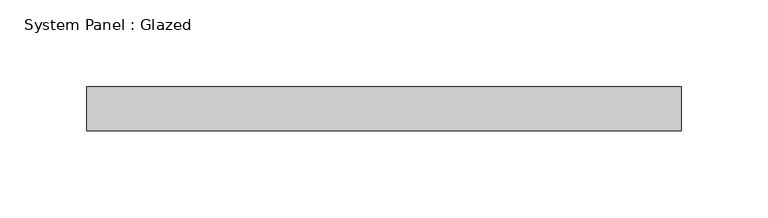
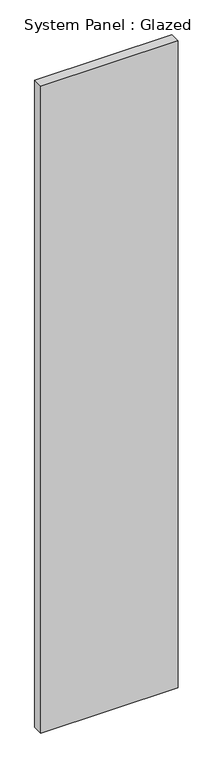
"""IFC4 building model written with IfcOpenShell, lengths in millimetres: plate geometry, System Panel : Glazed."""

from ifc_helpers import new_model, si_unit, origin, origin_with_axes, place, context, project, spatial, polyline, outline, extrude, source, transform, mapped, element, save


def system_panel_glazed_7c18a73f(model_context):
    return source(origin(), model_context, "Body", "SweptSolid", [
        extrude(outline(polyline([(171.45, 19.05), (-171.45, 19.05), (-171.45, 44.45), (171.45, 44.45), (171.45, 19.05)])), origin_with_axes(), (0.0, 0.0, 1.0), 1705.8927429),
    ])


if __name__ == "__main__":
    model = new_model("IFC4")
    model_context = context("Model", 3, world=origin())
    ifc_project = project(units=[si_unit("LENGTHUNIT", "METRE", prefix="MILLI")], contexts=[model_context])
    site = spatial("IfcSite", under=ifc_project)
    building = spatial("IfcBuilding", under=site)
    placement = place(None, origin())
    system_panel_glazed_shape = system_panel_glazed_7c18a73f(model_context)
    element("IfcPlate", 1, ObjectType="System Panel : Glazed", at=placement, inside=building, context=model_context, shape_type="MappedRepresentation", body=[
        mapped(system_panel_glazed_shape, transform((0.0, 0.0, 0.0), x_axis=(1.0, 0.0, 0.0), y_axis=(0.0, 1.0, 0.0), z_axis=(0.0, 0.0, 1.0))),
    ])
    save(model, "model.ifc")

# Revit data of these elements
# Type "System Panel : Glazed"
#   Construction Type Id = "GSP4R"
#   Analytic Construction = "1/8 in Pilkington single glazing"
#   Visual Light Transmittance = 0.9
#   Solar Heat Gain Coefficient = 0.86
#   Heat Transfer Coefficient (U) = 1.18115 BTU/(h·ft²·°F)
#   Define Thermal Properties by = 1
# Element 1 (IfcPlate, "System Panel : Glazed")
#   Materials on its faces: "Glass"
# Materials
#   "Glass": class "Glass", colour RGB 0 128 192, transparency 0.75, Description = "Soda Lime Glass", Cost = 0
